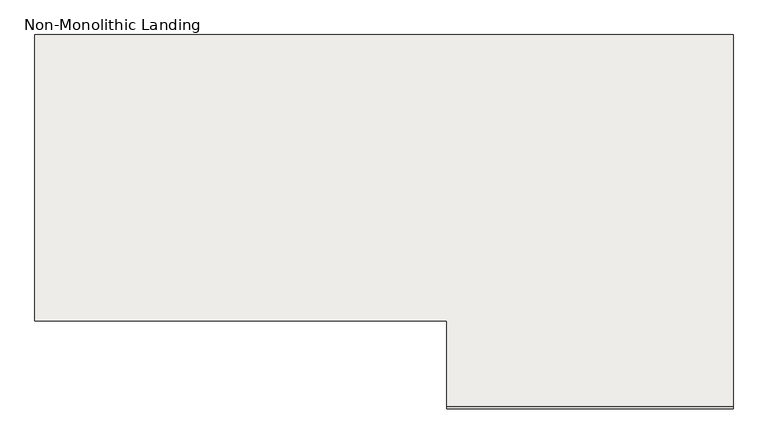
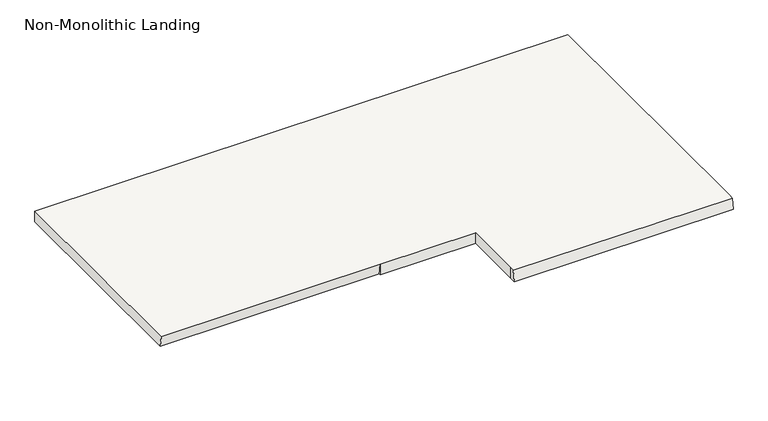
"""IFC4 building model written with IfcOpenShell, lengths in millimetres: slab geometry, Non-Monolithic Landing."""

from ifc_helpers import new_model, si_unit, origin, place, context, project, spatial, faceted_brep, source, transform, mapped, element, save


def non_monolithic_landing_ea8e6b74(model_context):
    return source(origin(), model_context, "Body", "Brep", [
        faceted_brep([(-10585.5805681, 2727.4280728, 1565.2173913), (-10585.5805681, 2720.2405728, 1515.2173913), (-9585.5547869, 2720.2405728, 1515.2173913), (-9585.5547869, 2727.4280728, 1565.2173913), (-11022.1547869, 3027.4280728, 1565.2173913), (-10585.5805681, 3027.4280728, 1565.2173913), (-10585.5805681, 2752.4280728, 1565.2173913), (-9585.5547869, 2752.4280728, 1565.2173913), (-9585.5547869, 4027.453854, 1565.2173913), (-12022.1805681, 4027.453854, 1565.2173913), (-12022.1805681, 3027.4280728, 1565.2173913), (-10585.5805681, 3027.4280728, 1515.2173913), (-11022.1547869, 3027.4280728, 1515.2173913), (-11022.1547869, 3034.6155728, 1515.2173913), (-12022.1805681, 3034.6155728, 1515.2173913), (-12022.1805681, 4027.453854, 1515.2173913), (-9585.5547869, 4027.453854, 1515.2173913), (-9585.5547869, 2752.4280728, 1515.2173913), (-10585.5805681, 2752.4280728, 1515.2173913)], [[[0, 1, 2, 3]], [[4, 5, 6, 0, 3, 7, 8, 9, 10]], [[11, 12, 13, 14, 15, 16, 17, 2, 1, 18]], [[5, 4, 12, 11]], [[6, 5, 11, 18]], [[0, 6, 18, 1]], [[7, 3, 2, 17]], [[8, 7, 17, 16]], [[9, 8, 16, 15]], [[10, 9, 15, 14]], [[4, 13, 12]], [[13, 4, 10, 14]]]),
    ])


if __name__ == "__main__":
    model = new_model("IFC4")
    model_context = context("Model", 3, world=origin())
    ifc_project = project(units=[si_unit("LENGTHUNIT", "METRE", prefix="MILLI")], contexts=[model_context])
    site = spatial("IfcSite", under=ifc_project)
    building = spatial("IfcBuilding", under=site)
    placement = place(None, origin())
    non_monolithic_landing_shape = non_monolithic_landing_ea8e6b74(model_context)
    element("IfcSlab", 1, ObjectType="Non-Monolithic Landing", at=placement, inside=building, context=model_context, shape_type="MappedRepresentation", body=[
        mapped(non_monolithic_landing_shape, transform((0.0, 0.0, 0.0), x_axis=(1.0, 0.0, 0.0), y_axis=(0.0, 1.0, 0.0), z_axis=(0.0, 0.0, 1.0))),
    ])
    save(model, "model.ifc")
